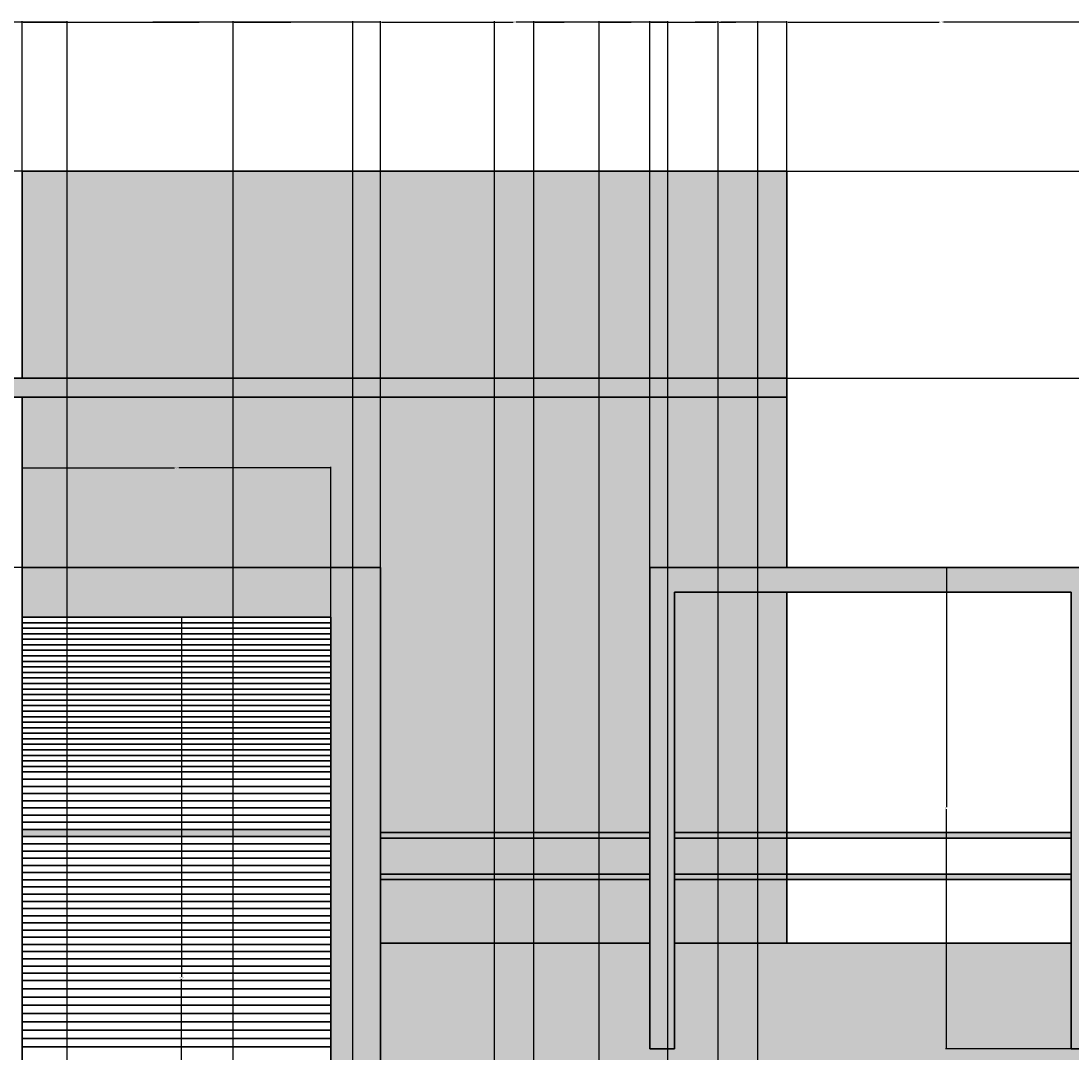
# Model space of a CAD drawing. Units: inches. Extents: x 73 to 607, y 92 to 651.
# Tile 16 of 18: x 256 to 446, y 465 to 651. Entities that reach past the tile are written whole.
import ezdxf

# ---------------------------------------------------------------- set-up
doc = ezdxf.new("R2010")
doc.units = ezdxf.units.IN
doc.header["$MEASUREMENT"] = 0
for name, color, linetype, lineweight in [('A-ANNO-DIMS', 2, 'Continuous', 18), ('A-ELEV', 7, 'Continuous', 35), ('A-ELEV-PATT-BKGD', 252, 'Continuous', 13), ('A-ELEV-PATT-STON', 42, 'Continuous', 13), ('A-ELEV-PATT-WALL', 254, 'Continuous', 13), ('A-ELEV-PATT-WOOD', 32, 'Continuous', 13), ('A-GLAZ-PATT', 7, 'Continuous', 13)]:
    doc.layers.add(name, color=color, linetype=linetype, lineweight=lineweight)
doc.styles.get("Standard").update_dxf_attribs({"font": 'arial.ttf'})
doc.dimstyles.get("Standard").update_dxf_attribs({"dimtxt": 0.18, "dimasz": 0.18, "dimexe": 0.18, "dimexo": 0.0625, "dimgap": 0.09, "dimtad": 0, "dimtih": 1, "dimtoh": 1, "dimdec": 4, "dimzin": 0, "dimdsep": 46, "dimtxsty": 'Standard', "dimcen": 0.09, "dimadec": 0, "dimazin": 0, "dimtfac": 1, "dimtdec": 4, "dimtofl": 0, "dimtmove": 0, "dimatfit": 3, "dimfxl": 1, "dimtolj": 1, "dimtzin": 0, "dimarcsym": 0})

# ---------------------------------------------------------------- blocks, each defined once
blk = doc.blocks.new('*D5')
at = {"layer": 'A-ANNO-DIMS', "color": 0, "lineweight": -2, "transparency": 16777216}
for p, q in [((256.41, 623.8), (72.92, 623.8)), ((73.1, 623.62), (73.1, 383.68)), ((73.1, 143.38), (73.1, 383.32)), ((100.04, 143.2), (72.92, 143.2))]:
    blk.add_line(p, q, dxfattribs=at)
at = {"layer": 'A-ANNO-DIMS', "color": 0, "transparency": 16777216}
for points in [[(73.07, 623.62), (73.13, 623.62), (73.1, 623.8)], [(73.07, 143.38), (73.13, 143.38), (73.1, 143.2)]]:
    blk.add_solid(points, dxfattribs=at)
at = {"layer": 'Defpoints', "color": 0, "transparency": 16777216}
for p in [(73.1, 623.8), (256.47, 623.8), (100.1, 143.2)]:
    blk.add_point(p, dxfattribs=at)
at = {"layer": 'A-ANNO-DIMS', "color": 0, "transparency": 16777216, "insert": (73.1, 383.5), "char_height": 0.18, "attachment_point": 5}
blk.add_mtext('\\A1;480.6', dxfattribs=at)
blk = doc.blocks.new('*D8')
at = {"layer": 'A-ANNO-DIMS', "color": 0, "lineweight": -2, "transparency": 16777216}
for p, q in [((229.32, 586.46), (229.32, 650.98)), ((229.5, 650.8), (242.43, 650.8)), ((256.29, 650.8), (243.36, 650.8)), ((256.47, 623.86), (256.47, 650.98))]:
    blk.add_line(p, q, dxfattribs=at)
at = {"layer": 'A-ANNO-DIMS', "color": 0, "transparency": 16777216}
for points in [[(229.5, 650.83), (229.5, 650.77), (229.32, 650.8)], [(256.29, 650.83), (256.29, 650.77), (256.47, 650.8)]]:
    blk.add_solid(points, dxfattribs=at)
at = {"layer": 'Defpoints', "color": 0, "transparency": 16777216}
for p in [(256.47, 650.8), (256.47, 623.8), (229.32, 586.39)]:
    blk.add_point(p, dxfattribs=at)
at = {"layer": 'A-ANNO-DIMS', "color": 0, "transparency": 16777216, "insert": (242.9, 650.8), "char_height": 0.18, "attachment_point": 5}
blk.add_mtext('\\A1;27.155', dxfattribs=at)
blk = doc.blocks.new('*D9')
at = {"layer": 'A-ANNO-DIMS', "color": 0, "lineweight": -2, "transparency": 16777216}
for p, q in [((256.47, 623.86), (256.47, 650.98)), ((256.65, 650.8), (288.49, 650.8)), ((321.12, 650.8), (289.28, 650.8)), ((321.3, 552.22), (321.3, 650.98))]:
    blk.add_line(p, q, dxfattribs=at)
at = {"layer": 'A-ANNO-DIMS', "color": 0, "transparency": 16777216}
for points in [[(256.65, 650.83), (256.65, 650.77), (256.47, 650.8)], [(321.12, 650.83), (321.12, 650.77), (321.3, 650.8)]]:
    blk.add_solid(points, dxfattribs=at)
at = {"layer": 'Defpoints', "color": 0, "transparency": 16777216}
for p in [(321.3, 650.8), (256.47, 623.8), (321.3, 552.16)]:
    blk.add_point(p, dxfattribs=at)
at = {"layer": 'A-ANNO-DIMS', "color": 0, "transparency": 16777216, "insert": (288.89, 650.8), "char_height": 0.18, "attachment_point": 5}
blk.add_mtext('\\A1;64.83', dxfattribs=at)
blk = doc.blocks.new('*D10')
at = {"layer": 'A-ANNO-DIMS', "color": 0, "lineweight": -2, "transparency": 16777216}
for p, q in [((321.3, 552.22), (321.3, 650.98)), ((321.48, 650.8), (345.24, 650.8)), ((369.79, 650.8), (346.03, 650.8)), ((369.97, 552.22), (369.97, 650.98))]:
    blk.add_line(p, q, dxfattribs=at)
at = {"layer": 'A-ANNO-DIMS', "color": 0, "transparency": 16777216}
for points in [[(321.48, 650.83), (321.48, 650.77), (321.3, 650.8)], [(369.79, 650.83), (369.79, 650.77), (369.97, 650.8)]]:
    blk.add_solid(points, dxfattribs=at)
at = {"layer": 'Defpoints', "color": 0, "transparency": 16777216}
for p in [(369.97, 650.8), (321.3, 552.16), (369.97, 552.16)]:
    blk.add_point(p, dxfattribs=at)
at = {"layer": 'A-ANNO-DIMS', "color": 0, "transparency": 16777216, "insert": (345.64, 650.8), "char_height": 0.18, "attachment_point": 5}
blk.add_mtext('\\A1;48.67', dxfattribs=at)
blk = doc.blocks.new('*D11')
at = {"layer": 'A-ANNO-DIMS', "color": 0, "lineweight": -2, "transparency": 16777216}
for p, q in [((369.97, 552.22), (369.97, 650.98)), ((370.15, 650.8), (381.91, 650.8)), ((394.6, 650.8), (382.84, 650.8)), ((394.78, 623.86), (394.78, 650.98))]:
    blk.add_line(p, q, dxfattribs=at)
at = {"layer": 'A-ANNO-DIMS', "color": 0, "transparency": 16777216}
for points in [[(370.15, 650.83), (370.15, 650.77), (369.97, 650.8)], [(394.6, 650.83), (394.6, 650.77), (394.78, 650.8)]]:
    blk.add_solid(points, dxfattribs=at)
at = {"layer": 'Defpoints', "color": 0, "transparency": 16777216}
for p in [(394.78, 650.8), (394.78, 623.8), (369.97, 552.16)]:
    blk.add_point(p, dxfattribs=at)
at = {"layer": 'A-ANNO-DIMS', "color": 0, "transparency": 16777216, "insert": (382.38, 650.8), "char_height": 0.18, "attachment_point": 5}
blk.add_mtext('\\A1;24.807', dxfattribs=at)
blk = doc.blocks.new('*D12')
at = {"layer": 'A-ANNO-DIMS', "color": 0, "lineweight": -2, "transparency": 16777216}
for p, q in [((394.78, 623.86), (394.78, 650.98)), ((394.96, 650.8), (422.33, 650.8)), ((450.48, 650.8), (423.11, 650.8)), ((450.66, 552.22), (450.66, 650.98))]:
    blk.add_line(p, q, dxfattribs=at)
at = {"layer": 'A-ANNO-DIMS', "color": 0, "transparency": 16777216}
for points in [[(394.96, 650.83), (394.96, 650.77), (394.78, 650.8)], [(450.48, 650.83), (450.48, 650.77), (450.66, 650.8)]]:
    blk.add_solid(points, dxfattribs=at)
at = {"layer": 'Defpoints', "color": 0, "transparency": 16777216}
for p in [(450.66, 650.8), (394.78, 623.8), (450.66, 552.16)]:
    blk.add_point(p, dxfattribs=at)
at = {"layer": 'A-ANNO-DIMS', "color": 0, "transparency": 16777216, "insert": (422.72, 650.8), "char_height": 0.18, "attachment_point": 5}
blk.add_mtext('\\A1;55.88', dxfattribs=at)
blk = doc.blocks.new('*D23')
at = {"layer": 'A-ANNO-DIMS', "color": 0, "lineweight": -2, "transparency": 16777216}
for p, q in [((394.84, 586.39), (607.28, 586.39)), ((607.1, 586.21), (607.1, 569.46)), ((607.1, 552.34), (607.1, 569.09)), ((580.16, 552.16), (607.28, 552.16))]:
    blk.add_line(p, q, dxfattribs=at)
at = {"layer": 'A-ANNO-DIMS', "color": 0, "transparency": 16777216}
for points in [[(607.07, 586.21), (607.13, 586.21), (607.1, 586.39)], [(607.07, 552.34), (607.13, 552.34), (607.1, 552.16)]]:
    blk.add_solid(points, dxfattribs=at)
at = {"layer": 'Defpoints', "color": 0, "transparency": 16777216}
for p in [(394.78, 586.39), (607.1, 586.39), (580.1, 552.16)]:
    blk.add_point(p, dxfattribs=at)
at = {"layer": 'A-ANNO-DIMS', "color": 0, "transparency": 16777216, "insert": (607.1, 569.28), "char_height": 0.18, "attachment_point": 5}
blk.add_mtext('\\A1;34.236', dxfattribs=at)
blk = doc.blocks.new('*D24')
at = {"layer": 'A-ANNO-DIMS', "color": 0, "lineweight": -2, "transparency": 16777216}
for p, q in [((394.84, 623.8), (607.28, 623.8)), ((607.1, 623.62), (607.1, 605.28)), ((607.1, 586.57), (607.1, 604.92)), ((394.84, 586.39), (607.28, 586.39))]:
    blk.add_line(p, q, dxfattribs=at)
at = {"layer": 'A-ANNO-DIMS', "color": 0, "transparency": 16777216}
for points in [[(607.07, 623.62), (607.13, 623.62), (607.1, 623.8)], [(607.07, 586.57), (607.13, 586.57), (607.1, 586.39)]]:
    blk.add_solid(points, dxfattribs=at)
at = {"layer": 'Defpoints', "color": 0, "transparency": 16777216}
for p in [(394.78, 623.8), (607.1, 623.8), (394.78, 586.39)]:
    blk.add_point(p, dxfattribs=at)
at = {"layer": 'A-ANNO-DIMS', "color": 0, "transparency": 16777216, "insert": (607.1, 605.1), "char_height": 0.18, "attachment_point": 5}
blk.add_mtext('\\A1;37.41', dxfattribs=at)
blk = doc.blocks.new('*D43')
at = {"layer": 'A-ANNO-DIMS', "color": 0, "lineweight": -2, "transparency": 16777216}
for p, q in [((256.47, 543.22), (256.47, 570.34)), ((256.65, 570.16), (283.99, 570.16)), ((312.12, 570.16), (284.78, 570.16)), ((312.3, 543.22), (312.3, 570.34))]:
    blk.add_line(p, q, dxfattribs=at)
at = {"layer": 'A-ANNO-DIMS', "color": 0, "transparency": 16777216}
for points in [[(256.65, 570.19), (256.65, 570.13), (256.47, 570.16)], [(312.12, 570.19), (312.12, 570.13), (312.3, 570.16)]]:
    blk.add_solid(points, dxfattribs=at)
at = {"layer": 'Defpoints', "color": 0, "transparency": 16777216}
for p in [(312.3, 570.16), (256.47, 543.16), (312.3, 543.16)]:
    blk.add_point(p, dxfattribs=at)
at = {"layer": 'A-ANNO-DIMS', "color": 0, "transparency": 16777216, "insert": (284.39, 570.16), "char_height": 0.18, "attachment_point": 5}
blk.add_mtext('\\A1;55.83', dxfattribs=at)
blk = doc.blocks.new('*D44')
at = {"layer": 'A-ANNO-DIMS', "color": 0, "lineweight": -2, "transparency": 16777216}
for p, q in [((312.24, 543.16), (285.12, 543.16)), ((285.3, 542.98), (285.3, 478.08)), ((285.3, 412.82), (285.3, 477.71)), ((312.24, 412.64), (285.12, 412.64))]:
    blk.add_line(p, q, dxfattribs=at)
at = {"layer": 'A-ANNO-DIMS', "color": 0, "transparency": 16777216}
for points in [[(285.27, 542.98), (285.33, 542.98), (285.3, 543.16)], [(285.27, 412.82), (285.33, 412.82), (285.3, 412.64)]]:
    blk.add_solid(points, dxfattribs=at)
at = {"layer": 'Defpoints', "color": 0, "transparency": 16777216}
for p in [(285.3, 543.16), (312.3, 543.16), (312.3, 412.64)]:
    blk.add_point(p, dxfattribs=at)
at = {"layer": 'A-ANNO-DIMS', "color": 0, "transparency": 16777216, "insert": (285.3, 477.9), "char_height": 0.18, "attachment_point": 5}
blk.add_mtext('\\A1;130.52', dxfattribs=at)
blk = doc.blocks.new('*D45')
at = {"layer": 'A-ANNO-DIMS', "color": 0, "lineweight": -2, "transparency": 16777216}
for p, q in [((256.41, 552.16), (229.29, 552.16)), ((229.47, 551.98), (229.47, 482.58)), ((229.47, 412.82), (229.47, 482.21)), ((256.41, 412.64), (229.29, 412.64))]:
    blk.add_line(p, q, dxfattribs=at)
at = {"layer": 'A-ANNO-DIMS', "color": 0, "transparency": 16777216}
for points in [[(229.44, 551.98), (229.5, 551.98), (229.47, 552.16)], [(229.44, 412.82), (229.5, 412.82), (229.47, 412.64)]]:
    blk.add_solid(points, dxfattribs=at)
at = {"layer": 'Defpoints', "color": 0, "transparency": 16777216}
for p in [(229.47, 552.16), (256.47, 552.16), (256.47, 412.64)]:
    blk.add_point(p, dxfattribs=at)
at = {"layer": 'A-ANNO-DIMS', "color": 0, "transparency": 16777216, "insert": (229.47, 482.4), "char_height": 0.18, "attachment_point": 5}
blk.add_mtext('\\A1;139.52', dxfattribs=at)
blk = doc.blocks.new('*D46')
at = {"layer": 'A-ANNO-DIMS', "color": 0, "lineweight": -2, "transparency": 16777216}
for p, q in [((450.6, 552.16), (423.48, 552.16)), ((423.66, 551.98), (423.66, 508.79)), ((423.66, 465.24), (423.66, 508.43)), ((450.6, 465.06), (423.48, 465.06))]:
    blk.add_line(p, q, dxfattribs=at)
at = {"layer": 'A-ANNO-DIMS', "color": 0, "transparency": 16777216}
for points in [[(423.63, 551.98), (423.69, 551.98), (423.66, 552.16)], [(423.63, 465.24), (423.69, 465.24), (423.66, 465.06)]]:
    blk.add_solid(points, dxfattribs=at)
at = {"layer": 'Defpoints', "color": 0, "transparency": 16777216}
for p in [(423.66, 552.16), (450.66, 552.16), (450.66, 465.06)]:
    blk.add_point(p, dxfattribs=at)
at = {"layer": 'A-ANNO-DIMS', "color": 0, "transparency": 16777216, "insert": (423.66, 508.61), "char_height": 0.18, "attachment_point": 5}
blk.add_mtext('\\A1;87.1', dxfattribs=at)
blk = doc.blocks.new('*D70')
at = {"layer": 'A-ANNO-DIMS', "color": 0, "lineweight": -2, "transparency": 16777216}
for p, q in [((241.43, 385.91), (241.43, 650.98)), ((241.61, 650.8), (252.54, 650.8)), ((264.41, 650.8), (253.47, 650.8)), ((264.59, 394.38), (264.59, 650.98))]:
    blk.add_line(p, q, dxfattribs=at)
at = {"layer": 'A-ANNO-DIMS', "color": 0, "transparency": 16777216}
for points in [[(241.61, 650.83), (241.61, 650.77), (241.43, 650.8)], [(264.41, 650.83), (264.41, 650.77), (264.59, 650.8)]]:
    blk.add_solid(points, dxfattribs=at)
at = {"layer": 'Defpoints', "color": 0, "transparency": 16777216}
for p in [(264.59, 650.8), (264.59, 394.31), (241.43, 385.85)]:
    blk.add_point(p, dxfattribs=at)
at = {"layer": 'A-ANNO-DIMS', "color": 0, "transparency": 16777216, "insert": (253.01, 650.8), "char_height": 0.18, "attachment_point": 5}
blk.add_mtext('\\A1;23.163', dxfattribs=at)
blk = doc.blocks.new('*D71')
at = {"layer": 'A-ANNO-DIMS', "color": 0, "lineweight": -2, "transparency": 16777216}
for p, q in [((264.59, 394.38), (264.59, 650.98)), ((264.77, 650.8), (279.15, 650.8)), ((294.46, 650.8), (280.08, 650.8)), ((294.64, 370.32), (294.64, 650.98))]:
    blk.add_line(p, q, dxfattribs=at)
at = {"layer": 'A-ANNO-DIMS', "color": 0, "transparency": 16777216}
for points in [[(264.77, 650.83), (264.77, 650.77), (264.59, 650.8)], [(294.46, 650.83), (294.46, 650.77), (294.64, 650.8)]]:
    blk.add_solid(points, dxfattribs=at)
at = {"layer": 'Defpoints', "color": 0, "transparency": 16777216}
for p in [(294.64, 650.8), (264.59, 394.31), (294.64, 370.25)]:
    blk.add_point(p, dxfattribs=at)
at = {"layer": 'A-ANNO-DIMS', "color": 0, "transparency": 16777216, "insert": (279.61, 650.8), "char_height": 0.18, "attachment_point": 5}
blk.add_mtext('\\A1;30.045', dxfattribs=at)
blk = doc.blocks.new('*D72')
at = {"layer": 'A-ANNO-DIMS', "color": 0, "lineweight": -2, "transparency": 16777216}
for p, q in [((294.64, 370.32), (294.64, 650.98)), ((294.82, 650.8), (305.06, 650.8)), ((316.1, 650.8), (305.86, 650.8)), ((316.28, 394.38), (316.28, 650.98))]:
    blk.add_line(p, q, dxfattribs=at)
at = {"layer": 'A-ANNO-DIMS', "color": 0, "transparency": 16777216}
for points in [[(294.82, 650.83), (294.82, 650.77), (294.64, 650.8)], [(316.1, 650.83), (316.1, 650.77), (316.28, 650.8)]]:
    blk.add_solid(points, dxfattribs=at)
at = {"layer": 'Defpoints', "color": 0, "transparency": 16777216}
for p in [(316.28, 650.8), (316.28, 394.31), (294.64, 370.25)]:
    blk.add_point(p, dxfattribs=at)
at = {"layer": 'A-ANNO-DIMS', "color": 0, "transparency": 16777216, "insert": (305.46, 650.8), "char_height": 0.18, "attachment_point": 5}
blk.add_mtext('\\A1;21.65', dxfattribs=at)
blk = doc.blocks.new('*D81')
at = {"layer": 'A-ANNO-DIMS', "color": 0, "lineweight": -2, "transparency": 16777216}
for p, q in [((341.87, 247.47), (341.87, 650.98)), ((342.05, 650.8), (345.04, 650.8)), ((348.82, 650.8), (345.83, 650.8)), ((349, 237.52), (349, 650.98))]:
    blk.add_line(p, q, dxfattribs=at)
at = {"layer": 'A-ANNO-DIMS', "color": 0, "transparency": 16777216}
for points in [[(342.05, 650.83), (342.05, 650.77), (341.87, 650.8)], [(348.82, 650.83), (348.82, 650.77), (349, 650.8)]]:
    blk.add_solid(points, dxfattribs=at)
at = {"layer": 'Defpoints', "color": 0, "transparency": 16777216}
for p in [(349, 650.8), (341.87, 247.41), (349, 237.45)]:
    blk.add_point(p, dxfattribs=at)
at = {"layer": 'A-ANNO-DIMS', "color": 0, "transparency": 16777216, "insert": (345.43, 650.8), "char_height": 0.18, "attachment_point": 5}
blk.add_mtext('\\A1;7.128', dxfattribs=at)
blk = doc.blocks.new('*D82')
at = {"layer": 'A-ANNO-DIMS', "color": 0, "lineweight": -2, "transparency": 16777216}
for p, q in [((349, 237.52), (349, 650.98)), ((349.18, 650.8), (354.47, 650.8)), ((360.67, 650.8), (355.38, 650.8)), ((360.85, 239), (360.85, 650.98))]:
    blk.add_line(p, q, dxfattribs=at)
at = {"layer": 'A-ANNO-DIMS', "color": 0, "transparency": 16777216}
for points in [[(349.18, 650.83), (349.18, 650.77), (349, 650.8)], [(360.67, 650.83), (360.67, 650.77), (360.85, 650.8)]]:
    blk.add_solid(points, dxfattribs=at)
at = {"layer": 'Defpoints', "color": 0, "transparency": 16777216}
for p in [(360.85, 650.8), (349, 237.45), (360.85, 238.93)]:
    blk.add_point(p, dxfattribs=at)
at = {"layer": 'A-ANNO-DIMS', "color": 0, "transparency": 16777216, "insert": (354.92, 650.8), "char_height": 0.18, "attachment_point": 5}
blk.add_mtext('\\A1;11.852', dxfattribs=at)
blk = doc.blocks.new('*D83')
at = {"layer": 'A-ANNO-DIMS', "color": 0, "lineweight": -2, "transparency": 16777216}
for p, q in [((360.85, 239), (360.85, 650.98)), ((361.03, 650.8), (366.6, 650.8)), ((373.08, 650.8), (367.51, 650.8)), ((373.26, 231.41), (373.26, 650.98))]:
    blk.add_line(p, q, dxfattribs=at)
at = {"layer": 'A-ANNO-DIMS', "color": 0, "transparency": 16777216}
for points in [[(361.03, 650.83), (361.03, 650.77), (360.85, 650.8)], [(373.08, 650.83), (373.08, 650.77), (373.26, 650.8)]]:
    blk.add_solid(points, dxfattribs=at)
at = {"layer": 'Defpoints', "color": 0, "transparency": 16777216}
for p in [(373.26, 650.8), (360.85, 238.93), (373.26, 231.35)]:
    blk.add_point(p, dxfattribs=at)
at = {"layer": 'A-ANNO-DIMS', "color": 0, "transparency": 16777216, "insert": (367.05, 650.8), "char_height": 0.18, "attachment_point": 5}
blk.add_mtext('\\A1;12.408', dxfattribs=at)
blk = doc.blocks.new('*D84')
at = {"layer": 'A-ANNO-DIMS', "color": 0, "lineweight": -2, "transparency": 16777216}
for p, q in [((373.26, 231.41), (373.26, 650.98)), ((373.44, 650.8), (377.4, 650.8)), ((382.15, 650.8), (378.19, 650.8)), ((382.33, 241.03), (382.33, 650.98))]:
    blk.add_line(p, q, dxfattribs=at)
at = {"layer": 'A-ANNO-DIMS', "color": 0, "transparency": 16777216}
for points in [[(373.44, 650.83), (373.44, 650.77), (373.26, 650.8)], [(382.15, 650.83), (382.15, 650.77), (382.33, 650.8)]]:
    blk.add_solid(points, dxfattribs=at)
at = {"layer": 'Defpoints', "color": 0, "transparency": 16777216}
for p in [(382.33, 650.8), (382.33, 240.97), (373.26, 231.35)]:
    blk.add_point(p, dxfattribs=at)
at = {"layer": 'A-ANNO-DIMS', "color": 0, "transparency": 16777216, "insert": (377.79, 650.8), "char_height": 0.18, "attachment_point": 5}
blk.add_mtext('\\A1;9.074', dxfattribs=at)
blk = doc.blocks.new('*D85')
at = {"layer": 'A-ANNO-DIMS', "color": 0, "lineweight": -2, "transparency": 16777216}
for p, q in [((382.33, 241.03), (382.33, 650.98)), ((382.51, 650.8), (385.55, 650.8)), ((389.37, 650.8), (386.33, 650.8)), ((389.55, 232.52), (389.55, 650.98))]:
    blk.add_line(p, q, dxfattribs=at)
at = {"layer": 'A-ANNO-DIMS', "color": 0, "transparency": 16777216}
for points in [[(382.51, 650.83), (382.51, 650.77), (382.33, 650.8)], [(389.37, 650.83), (389.37, 650.77), (389.55, 650.8)]]:
    blk.add_solid(points, dxfattribs=at)
at = {"layer": 'Defpoints', "color": 0, "transparency": 16777216}
for p in [(389.55, 650.8), (382.33, 240.97), (389.55, 232.46)]:
    blk.add_point(p, dxfattribs=at)
at = {"layer": 'A-ANNO-DIMS', "color": 0, "transparency": 16777216, "insert": (385.94, 650.8), "char_height": 0.18, "attachment_point": 5}
blk.add_mtext('\\A1;7.222', dxfattribs=at)

msp = doc.modelspace()

# ---------------------------------------------------------------- hatches: boundary and pattern name
at = {"layer": 'A-ELEV-PATT-BKGD'}
h = msp.add_hatch(color=256, dxfattribs=at)
h.dxf.hatch_style = 1
h.paths.add_polyline_path([(321.3008, 479.2042), (312.3008, 479.2042), (312.3008, 478.7576), (312.3008, 412.636), (321.3008, 412.636)])
h.paths.add_polyline_path([(312.3008, 504.7576), (256.4726, 504.7576), (256.4726, 503.4576), (312.3008, 503.4576)], flags=17)
h.paths.add_polyline_path([(321.3008, 543.1576), (321.3008, 552.1576), (320.3257, 552.1576), (312.3008, 552.1576), (256.4726, 552.1576), (256.4726, 543.1576), (312.3008, 543.1576), (312.3008, 479.2042), (321.3008, 479.2042)])
h.paths.add_polyline_path([(451.5214, 412.636), (256.4726, 412.636), (256.4726, 403.636), (442.5214, 403.636), (442.5214, 320.2042), (206.1343, 320.2042), (206.1343, 320.9135), (206.1343, 403.636), (256.4726, 403.636), (256.4726, 412.636), (201.6343, 412.636), (201.6343, 320.9135), (201.6343, 320.2042), (201.6343, 311.2042), (256.4726, 311.2042), (451.5214, 311.2042)])
h.paths.add_polyline_path([(431.07, 258.6914), (369.5339, 258.6914), (369.5339, 247.4054), (396.692, 247.4054), (425.07, 247.4054), (425.07, 194.7312), (396.692, 194.6197), (396.692, 194.5366), (369.5339, 194.5366), (369.5339, 185.6619), (431.07, 185.6619)])
h.paths.add_polyline_path([(580.0983, 262.3024), (451.5214, 262.3024), (451.5214, 143.2042), (580.0983, 143.2042)])
h.paths.add_polyline_path([(454.7049, 174.802), (454.7049, 256.6321), (577.9249, 256.6321), (577.9249, 174.802)], flags=16)
h.paths.add_polyline_path([(465.9716, 191.1416, -1), (473.7874, 191.1416, -1)], flags=0)
h.paths.add_polyline_path([(490.5373, 181.6586, -1), (494.9999, 181.6586, -1)], flags=0)
h.paths.add_polyline_path([(476.2996, 209.8287, -1), (500.5844, 209.8287, -1)], flags=0)
h.paths.add_polyline_path([(505.3326, 194.7675, -1), (512.5843, 194.7675, -1)], flags=0)
h.paths.add_polyline_path([(520.9613, 186.679, -1), (526.544, 186.679, -1)], flags=0)
h.paths.add_polyline_path([(466.8103, 225.7267, -1), (470.1573, 225.7267, -1)], flags=0)
h.paths.add_polyline_path([(527.1059, 203.6926, -1), (536.0311, 203.6926, -1)], flags=0)
h.paths.add_polyline_path([(504.775, 232.6995, -1), (513.7002, 232.6995, -1)], flags=0)
h.paths.add_polyline_path([(546.9241, 183.611, -1), (554.7336, 183.611, -1)], flags=0)
h.paths.add_polyline_path([(459.5544, 243.856, -1), (466.8061, 243.856, -1)], flags=0)
h.paths.add_polyline_path([(476.3045, 246.924, -1), (488.5767, 246.924, -1)], flags=0)
h.paths.add_polyline_path([(529.9044, 226.8424, -1), (556.68, 226.8424, -1)], flags=0)
h.paths.add_polyline_path([(554.1814, 203.9716, -1), (561.4331, 203.9716, -1)], flags=0)
h.paths.add_polyline_path([(567.8561, 193.3729, -1), (570.6475, 193.3729, -1)], flags=0)
h.paths.add_polyline_path([(522.3584, 250.271, -1), (525.7053, 250.271, -1)], flags=0)
h.paths.add_polyline_path([(561.9965, 245.2506, -1), (567.5748, 245.2506, -1)], flags=0)
h.paths.add_polyline_path([(347.8686, 194.5366), (341.8686, 194.5366), (341.8686, 194.5452), (314.0144, 194.5452), (314.0144, 188.5452), (347.8686, 188.5452)])
h.paths.add_polyline_path([(347.8686, 253.4054), (314.0144, 253.4054), (314.0144, 247.4054), (341.8686, 247.4054), (347.8686, 247.4054)])
h.paths.add_polyline_path([(304.3559, 253.4054), (298.3559, 253.4054), (298.3559, 188.5452), (304.3559, 188.5452)])
h.paths.add_polyline_path([(450.6603, 552.1576), (369.9727, 552.1576), (369.9727, 479.2042), (374.4727, 479.2042), (374.4727, 547.6576), (446.1603, 547.6576), (446.1603, 479.2042), (450.6603, 479.2042)])
h.paths.add_polyline_path([(374.4727, 479.2042), (369.9727, 479.2042), (369.9727, 465.0632), (374.4727, 465.0632)])
h.paths.add_polyline_path([(450.6603, 479.2042), (446.1603, 479.2042), (446.1603, 465.0632), (450.6603, 465.0632)])
h.paths.add_polyline_path([(256.4726, 281.6039), (109.0983, 281.6039), (100.0983, 281.6039), (100.0983, 167.2042), (100.0983, 143.2042), (109.0983, 143.2042), (109.0983, 167.2042), (109.0983, 272.6039), (256.4726, 272.6039)])
at = {"layer": 'A-ELEV-PATT-STON'}
h = msp.add_hatch(color=256, dxfattribs=at)
h.dxf.hatch_style = 1
h.paths.add_polyline_path([(394.7799, 623.801), (256.4726, 623.801), (256.4726, 586.3933), (394.7799, 586.3933)])
h.paths.add_polyline_path([(233.924, 582.9721), (229.3177, 582.9721), (229.3177, 412.636), (233.924, 412.636)])
h.paths.add_polyline_path([(234.1465, 311.2042), (229.0534, 311.2042), (229.0534, 281.6039), (234.1465, 281.6039)])
h.paths.add_polyline_path([(234.384, 272.6039), (228.8076, 272.6039), (228.8076, 167.2042), (234.384, 167.2042)])
h = msp.add_hatch(color=256, dxfattribs=at)
h.dxf.hatch_style = 1
h.paths.add_polyline_path([(394.7799, 582.9721), (256.4726, 582.9721), (256.4726, 552.1576), (312.3008, 552.1576), (320.3257, 552.1576), (321.3008, 552.1576), (321.3008, 543.1576), (321.3008, 504.2042), (369.9727, 504.2042), (369.9727, 552.1576), (394.7799, 552.1576)])
h = msp.add_hatch(color=256, dxfattribs=at)
h.dxf.hatch_style = 1
h.paths.add_polyline_path([(394.7799, 547.6576), (374.4727, 547.6576), (374.4727, 504.2042), (394.7799, 504.2042)])
h = msp.add_hatch(color=256, dxfattribs=at)
h.dxf.hatch_style = 1
h.paths.add_polyline_path([(394.7799, 503.2042), (374.4727, 503.2042), (374.4727, 496.6899), (394.7799, 496.6899)])
h.paths.add_polyline_path([(394.7799, 495.6899), (374.4727, 495.6899), (374.4727, 484.2142), (394.7799, 484.2142)])
h.paths.add_polyline_path([(369.9727, 495.6899), (321.3008, 495.6899), (321.3008, 484.2142), (369.9727, 484.2142)])
h.paths.add_polyline_path([(369.9727, 503.2042), (321.3008, 503.2042), (321.3008, 496.6899), (369.9727, 496.6899)])
at = {"layer": 'A-ELEV-PATT-WALL'}
h = msp.add_hatch(color=256, dxfattribs=at)
h.dxf.hatch_style = 1
h.paths.add_polyline_path([(509.9692, 483.857), (450.6603, 483.857), (450.6603, 465.0632), (446.1603, 465.0632), (446.1603, 484.2142), (374.4727, 484.2142), (374.4727, 465.0632), (369.9727, 465.0632), (369.9727, 484.2142), (321.3008, 484.2142), (321.3008, 412.636), (451.5214, 412.636), (451.5214, 311.2042), (314.0144, 311.2042), (314.0144, 253.4054), (347.8686, 253.4054), (347.8686, 247.4054), (369.5339, 247.4054), (369.5339, 258.6914), (431.07, 258.6914), (431.07, 185.6619), (369.5339, 185.6619), (369.5339, 194.5366), (347.8686, 194.5366), (347.8686, 188.5452), (314.0144, 188.5452), (314.0144, 143.2042), (451.5214, 143.2042), (451.5214, 262.3024), (580.0983, 262.3024), (580.0983, 311.2042), (509.9692, 311.2042)])
h.paths.add_polyline_path([(304.3559, 311.2042), (256.4726, 311.2042), (256.4726, 167.2042), (256.4726, 143.2042), (304.3559, 143.2042), (304.3559, 188.5452), (298.3559, 188.5452), (298.3559, 253.4054), (304.3559, 253.4054)])
at = {"layer": 'A-ELEV-PATT-WOOD'}
h = msp.add_hatch(color=256, dxfattribs=at)
h.dxf.hatch_style = 1
h.paths.add_polyline_path([(394.7799, 586.3933), (229.3177, 586.3933), (229.3177, 582.9721), (394.7799, 582.9721)])
at = {"layer": 'A-GLAZ-PATT'}
h = msp.add_hatch(color=256, dxfattribs=at)
h.dxf.hatch_style = 1
h.paths.add_polyline_path([(369.9727, 496.6899), (321.3008, 496.6899), (321.3008, 495.6899), (369.9727, 495.6899)])
h.paths.add_polyline_path([(394.7799, 496.6899), (374.4727, 496.6899), (374.4727, 495.6899), (394.7799, 495.6899)])
h.paths.add_polyline_path([(446.1603, 496.6899), (394.7799, 496.6899), (394.7799, 495.6899), (446.1603, 495.6899)])
h.paths.add_polyline_path([(446.1603, 504.2042), (394.7799, 504.2042), (394.7799, 503.2042), (446.1603, 503.2042)])
h.paths.add_polyline_path([(369.9727, 504.2042), (321.3008, 504.2042), (321.3008, 503.2042), (369.9727, 503.2042)])
h.paths.add_polyline_path([(394.7799, 504.2042), (374.4727, 504.2042), (374.4727, 503.2042), (394.7799, 503.2042)])
h.paths.add_polyline_path([(509.9692, 504.2042), (450.6603, 504.2042), (450.6603, 503.2042), (509.9692, 503.2042)])
h.paths.add_polyline_path([(509.9692, 496.6899), (450.6603, 496.6899), (450.6603, 495.6899), (509.9692, 495.6899)])
h.paths.add_polyline_path([(409.515, 342.1009), (338.6695, 342.1009), (338.6695, 341.1009), (409.515, 341.1009)])
h.paths.add_polyline_path([(442.5214, 338.0025), (338.6695, 338.0025), (338.6695, 337.0025), (442.5214, 337.0025)])
h.paths.add_polyline_path([(442.5214, 332.9397), (338.6695, 332.9397), (338.6695, 331.9397), (442.5214, 331.9397)])

# ---------------------------------------------------------------- linework, layer by layer
at = {"layer": 'A-ELEV'}
for p, q in [((256.4726, 586.3933), (256.4726, 623.801)), ((256.4726, 623.801), (394.7799, 623.801)), ((394.7799, 623.801), (394.7799, 552.1576)), ((256.4726, 582.9721), (256.4726, 552.1576)), ((312.3008, 552.1576), (256.4726, 552.1576)), ((256.4726, 552.1576), (256.4726, 542.7562)), ((320.3257, 552.1576), (312.3008, 552.1576)), ((321.3008, 552.1576), (320.3257, 552.1576)), ((321.3008, 543.1576), (321.3008, 552.1576)), ((369.9727, 465.0632), (369.9727, 552.1576)), ((369.9727, 552.1576), (450.6603, 552.1576)), ((374.4727, 465.0632), (374.4727, 547.6576)), ((374.4727, 547.6576), (446.1603, 547.6576)), ((394.7799, 547.6576), (394.7799, 484.2142)), ((446.1603, 547.6576), (446.1603, 465.0632)), ((312.3008, 543.1576), (256.4726, 543.1576)), ((256.4726, 543.1576), (256.4726, 503.2042)), ((312.3008, 412.636), (312.3008, 543.1576)), ((321.3008, 412.636), (321.3008, 543.1576)), ((312.3008, 542.1576), (256.4726, 542.1576)), ((312.3008, 541.1576), (256.4726, 541.1576)), ((312.3008, 540.1576), (256.4726, 540.1576)), ((312.3008, 539.1576), (256.4726, 539.1576)), ((312.3008, 538.1576), (256.4726, 538.1576)), ((312.3008, 537.1576), (256.4726, 537.1576)), ((312.3008, 536.1576), (256.4726, 536.1576)), ((312.3008, 535.1576), (256.4726, 535.1576)), ((312.3008, 534.1576), (256.4726, 534.1576)), ((312.3008, 533.1576), (256.4726, 533.1576)), ((312.3008, 532.1576), (256.4726, 532.1576)), ((312.3008, 531.1576), (256.4726, 531.1576)), ((312.3008, 530.1576), (256.4726, 530.1576)), ((312.3008, 529.1576), (256.4726, 529.1576)), ((312.3008, 528.1576), (256.4726, 528.1576)), ((312.3008, 527.1576), (256.4726, 527.1576)), ((312.3008, 526.1576), (256.4726, 526.1576)), ((312.3008, 525.1576), (256.4726, 525.1576)), ((312.3008, 524.1576), (256.4726, 524.1576)), ((312.3008, 523.1576), (256.4726, 523.1576)), ((312.3008, 522.1576), (256.4726, 522.1576)), ((312.3008, 521.1576), (256.4726, 521.1576)), ((312.3008, 520.1576), (256.4726, 520.1576)), ((312.3008, 519.1576), (256.4726, 519.1576)), ((312.3008, 518.1576), (256.4726, 518.1576)), ((312.3008, 517.1576), (256.4726, 517.1576)), ((312.3008, 516.1576), (256.4726, 516.1576)), ((312.3008, 515.1576), (256.4726, 515.1576)), ((312.3008, 513.8576), (256.4726, 513.8576)), ((312.3008, 512.5576), (256.4726, 512.5576)), ((312.3008, 511.2576), (256.4726, 511.2576)), ((312.3008, 509.9576), (256.4726, 509.9576)), ((312.3008, 508.6576), (256.4726, 508.6576)), ((312.3008, 507.3576), (256.4726, 507.3576)), ((312.3008, 506.0576), (256.4726, 506.0576)), ((312.3008, 504.7576), (256.4726, 504.7576)), ((312.3008, 503.4576), (256.4726, 503.4576)), ((321.3008, 504.2042), (369.9727, 504.2042)), ((374.4727, 504.2042), (446.1603, 504.2042)), ((256.4726, 455.2042), (256.4726, 503.2042)), ((312.3008, 502.1576), (256.4726, 502.1576)), ((321.3008, 503.2042), (369.9727, 503.2042)), ((374.4727, 503.2042), (446.1603, 503.2042)), ((312.3008, 500.8576), (256.4726, 500.8576)), ((312.3008, 499.5576), (256.4726, 499.5576)), ((312.3008, 498.2576), (256.4726, 498.2576)), ((312.3008, 496.9576), (256.4726, 496.9576)), ((312.3008, 495.6576), (256.4726, 495.6576)), ((321.3008, 496.6899), (369.9727, 496.6899)), ((321.3008, 495.6899), (369.9727, 495.6899)), ((374.4727, 496.6899), (446.1603, 496.6899)), ((374.4727, 495.6899), (446.1603, 495.6899)), ((312.3008, 494.3576), (256.4726, 494.3576)), ((312.3008, 493.0576), (256.4726, 493.0576)), ((312.3008, 491.7576), (256.4726, 491.7576)), ((312.3008, 490.4576), (256.4726, 490.4576)), ((312.3008, 489.1576), (256.4726, 489.1576)), ((312.3008, 487.8576), (256.4726, 487.8576)), ((312.3008, 486.5576), (256.4726, 486.5576)), ((312.3008, 485.2576), (256.4726, 485.2576)), ((312.3008, 483.9576), (256.4726, 483.9576)), ((312.3008, 482.6576), (256.4726, 482.6576)), ((321.3008, 484.2142), (369.9727, 484.2142)), ((374.4727, 484.2142), (446.1603, 484.2142)), ((312.3008, 481.3576), (256.4726, 481.3576)), ((312.3008, 480.0576), (256.4726, 480.0576)), ((312.3008, 478.7576), (256.4726, 478.7576)), ((312.3008, 477.4576), (256.4726, 477.4576)), ((312.3008, 475.9576), (256.4726, 475.9576)), ((312.3008, 474.4576), (256.4726, 474.4576)), ((312.3008, 472.9576), (256.4726, 472.9576)), ((312.3008, 471.4576), (256.4726, 471.4576)), ((312.3008, 469.9576), (256.4726, 469.9576)), ((312.3008, 468.4576), (256.4726, 468.4576)), ((312.3008, 466.9576), (256.4726, 466.9576)), ((312.3008, 465.4576), (256.4726, 465.4576)), ((369.9727, 465.0632), (374.4727, 465.0632)), ((446.1603, 465.0632), (450.6603, 465.0632))]:
    msp.add_line(p, q, dxfattribs=at)
msp.add_lwpolyline([(229.3177, 582.9721), (394.7799, 582.9721), (394.7799, 586.3933), (229.3177, 586.3933)], close=True, dxfattribs=at)

# ---------------------------------------------------------------- dimensions: what is measured, and where the dimension line sits
at = {"layer": 'A-ANNO-DIMS'}
for base, p1, p2, override, picture, middle in [((256.4726, 650.801), (229.3177, 586.3933), (256.4726, 623.801), {"dimdec": 3, "dimlfac": 1, "dimrnd": 0, "dimzin": 0, "dimdsep": 46, "dimlunit": 2}, '*D8', (242.8951, 650.801)), ((264.5904, 650.801), (241.4273, 385.8466), (264.5904, 394.3141), {"dimdec": 3, "dimlfac": 1, "dimrnd": 0, "dimzin": 0, "dimdsep": 46, "dimlunit": 2}, '*D70', (253.0088, 650.801)), ((321.3008, 650.801), (256.4726, 623.801), (321.3008, 552.1576), {"dimdec": 2, "dimlfac": 1, "dimrnd": 0, "dimzin": 0, "dimdsep": 46, "dimlunit": 2}, '*D9', (288.8867, 650.801)), ((294.6352, 650.801), (264.5904, 394.3141), (294.6352, 370.2541), {"dimdec": 3, "dimlfac": 1, "dimrnd": 0, "dimzin": 0, "dimdsep": 46, "dimlunit": 2}, '*D71', (279.6128, 650.801)), ((316.2836, 650.801), (294.6352, 370.2541), (316.2836, 394.3141), {"dimdec": 2, "dimlfac": 1, "dimrnd": 0, "dimzin": 0, "dimdsep": 46, "dimlunit": 2}, '*D72', (305.4594, 650.801)), ((369.9727, 650.801), (321.3008, 552.1576), (369.9727, 552.1576), {"dimdec": 2, "dimlfac": 1, "dimrnd": 0, "dimzin": 0, "dimdsep": 46, "dimlunit": 2}, '*D10', (345.6367, 650.801)), ((348.9968, 650.801), (341.8686, 247.4054), (348.9968, 237.4546), {"dimdec": 3, "dimlfac": 1, "dimrnd": 0, "dimzin": 0, "dimdsep": 46, "dimlunit": 2}, '*D81', (345.4327, 650.801)), ((360.8489, 650.801), (348.9968, 237.4546), (360.8489, 238.9349), {"dimdec": 3, "dimlfac": 1, "dimrnd": 0, "dimzin": 0, "dimdsep": 46, "dimlunit": 2}, '*D82', (354.9229, 650.801)), ((373.2566, 650.801), (360.8489, 238.9349), (373.2566, 231.3482), {"dimdec": 3, "dimlfac": 1, "dimrnd": 0, "dimzin": 0, "dimdsep": 46, "dimlunit": 2}, '*D83', (367.0527, 650.801)), ((394.7799, 650.801), (369.9727, 552.1576), (394.7799, 623.801), {"dimdec": 3, "dimlfac": 1, "dimrnd": 0, "dimzin": 0, "dimdsep": 46, "dimlunit": 2}, '*D11', (382.3763, 650.801)), ((382.3308, 650.801), (373.2566, 231.3482), (382.3308, 240.9703), {"dimdec": 3, "dimlfac": 1, "dimrnd": 0, "dimzin": 0, "dimdsep": 46, "dimlunit": 2}, '*D84', (377.7937, 650.801)), ((389.5532, 650.801), (382.3308, 240.9703), (389.5532, 232.4585), {"dimdec": 3, "dimlfac": 1, "dimrnd": 0, "dimzin": 0, "dimdsep": 46, "dimlunit": 2}, '*D85', (385.942, 650.801)), ((450.6603, 650.801), (394.7799, 623.801), (450.6603, 552.1576), {"dimdec": 2, "dimlfac": 1, "dimrnd": 0, "dimzin": 0, "dimdsep": 46, "dimlunit": 2}, '*D12', (422.7201, 650.801)), ((312.3008, 570.1576), (256.4726, 543.1576), (312.3008, 543.1576), {"dimdec": 2, "dimlfac": 1, "dimrnd": 0, "dimzin": 0, "dimdsep": 46, "dimlunit": 2}, '*D43', (284.3867, 570.1576))]:
    dim = msp.add_linear_dim(base=base, p1=p1, p2=p2, dimstyle='Standard', override=override, dxfattribs=at)
    dim.commit()
    dim.dimension.update_dxf_attribs({"geometry": picture, "text_midpoint": middle})
for base, p1, p2, override, picture, middle in [((73.0983, 623.801), (100.0983, 143.2042), (256.4726, 623.801), {"dimdec": 1, "dimlfac": 1, "dimrnd": 0, "dimzin": 0, "dimdsep": 46, "dimlunit": 2}, '*D5', (73.0983, 383.5026)), ((607.0983, 623.801), (394.7799, 586.3933), (394.7799, 623.801), {"dimdec": 2, "dimlfac": 1, "dimrnd": 0, "dimzin": 0, "dimdsep": 46, "dimlunit": 2}, '*D24', (607.0983, 605.0972)), ((607.0983, 586.3933), (580.0983, 552.1576), (394.7799, 586.3933), {"dimdec": 3, "dimlfac": 1, "dimrnd": 0, "dimzin": 0, "dimdsep": 46, "dimlunit": 2}, '*D23', (607.0983, 569.2755)), ((229.4726, 552.1576), (256.4726, 412.636), (256.4726, 552.1576), {"dimdec": 2, "dimlfac": 1, "dimrnd": 0, "dimzin": 0, "dimdsep": 46, "dimlunit": 2}, '*D45', (229.4726, 482.3968)), ((423.6603, 552.1576), (450.6603, 465.0632), (450.6603, 552.1576), {"dimdec": 1, "dimlfac": 1, "dimrnd": 0, "dimzin": 0, "dimdsep": 46, "dimlunit": 2}, '*D46', (423.6603, 508.6104)), ((285.3008, 543.1576), (312.3008, 412.636), (312.3008, 543.1576), {"dimdec": 2, "dimlfac": 1, "dimrnd": 0, "dimzin": 0, "dimdsep": 46, "dimlunit": 2}, '*D44', (285.3008, 477.8968))]:
    dim = msp.add_linear_dim(base=base, p1=p1, p2=p2, angle=90, dimstyle='Standard', override=override, dxfattribs=at)
    dim.commit()
    dim.dimension.update_dxf_attribs({"geometry": picture, "text_midpoint": middle})

doc.saveas('drawing.dxf')
